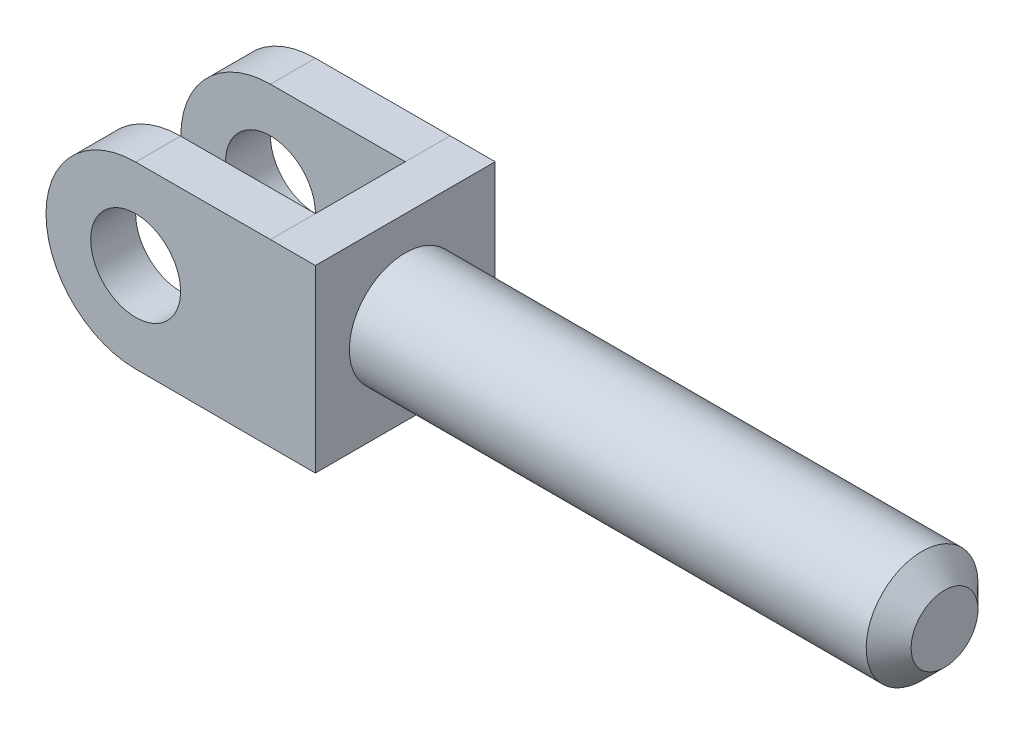
ISO-10303-21;
HEADER;
FILE_DESCRIPTION(('STEP AP214'),'2;1');
FILE_NAME('part.step','',(''),(''),'','','');
FILE_SCHEMA(('AUTOMOTIVE_DESIGN { 1 0 10303 214 1 1 1 1 }'));
ENDSEC;
DATA;
#1=APPLICATION_CONTEXT('core data for automotive mechanical design processes');
#2=APPLICATION_PROTOCOL_DEFINITION('international standard','automotive_design',2000,#1);
#3=PRODUCT_CONTEXT('',#1,'mechanical');
#4=PRODUCT('Part','Part','',(#3));
#5=PRODUCT_RELATED_PRODUCT_CATEGORY('part','',(#4));
#6=PRODUCT_DEFINITION_FORMATION('','',#4);
#7=PRODUCT_DEFINITION_CONTEXT('part definition',#1,'design');
#8=PRODUCT_DEFINITION('design','',#6,#7);
#9=PRODUCT_DEFINITION_SHAPE('','',#8);
#10=(LENGTH_UNIT() NAMED_UNIT(*) SI_UNIT(.MILLI.,.METRE.));
#11=(NAMED_UNIT(*) PLANE_ANGLE_UNIT() SI_UNIT($,.RADIAN.));
#12=(NAMED_UNIT(*) SI_UNIT($,.STERADIAN.) SOLID_ANGLE_UNIT());
#13=UNCERTAINTY_MEASURE_WITH_UNIT(LENGTH_MEASURE(1.E-05),#10,'distance_accuracy_value','');
#14=(GEOMETRIC_REPRESENTATION_CONTEXT(3) GLOBAL_UNCERTAINTY_ASSIGNED_CONTEXT((#13)) GLOBAL_UNIT_ASSIGNED_CONTEXT((#10,
#11,#12)) REPRESENTATION_CONTEXT('',''));
#15=CARTESIAN_POINT('',(0.,0.,0.));
#16=DIRECTION('',(0.,0.,1.));
#17=DIRECTION('',(1.,0.,0.));
#18=AXIS2_PLACEMENT_3D('',#15,#16,#17);
#19=CARTESIAN_POINT('',(0.,6.35,6.35));
#20=DIRECTION('',(1.,0.,0.));
#21=DIRECTION('',(0.,1.,0.));
#22=AXIS2_PLACEMENT_3D('',#19,#20,#21);
#23=PLANE('',#22);
#24=DIRECTION('',(0.,-1.,0.));
#25=VECTOR('',#24,1.);
#26=CARTESIAN_POINT('',(0.,6.35,3.175));
#27=LINE('',#26,#25);
#28=CARTESIAN_POINT('',(0.,6.35,3.175));
#29=VERTEX_POINT('',#28);
#30=CARTESIAN_POINT('',(0.,-6.35,3.175));
#31=VERTEX_POINT('',#30);
#32=EDGE_CURVE('E136',#29,#31,#27,.T.);
#33=ORIENTED_EDGE('',*,*,#32,.F.);
#34=DIRECTION('',(0.,0.,-1.));
#35=VECTOR('',#34,1.);
#36=CARTESIAN_POINT('',(0.,6.35,6.35));
#37=LINE('',#36,#35);
#38=CARTESIAN_POINT('',(0.,6.35,-3.175));
#39=VERTEX_POINT('',#38);
#40=EDGE_CURVE('E211',#29,#39,#37,.T.);
#41=ORIENTED_EDGE('',*,*,#40,.T.);
#42=DIRECTION('',(0.,-1.,0.));
#43=VECTOR('',#42,1.);
#44=CARTESIAN_POINT('',(0.,6.35,-3.175));
#45=LINE('',#44,#43);
#46=CARTESIAN_POINT('',(0.,-6.35,-3.175));
#47=VERTEX_POINT('',#46);
#48=EDGE_CURVE('E179',#39,#47,#45,.T.);
#49=ORIENTED_EDGE('',*,*,#48,.T.);
#50=DIRECTION('',(0.,0.,-1.));
#51=VECTOR('',#50,1.);
#52=CARTESIAN_POINT('',(0.,-6.35,6.35));
#53=LINE('',#52,#51);
#54=EDGE_CURVE('E60',#31,#47,#53,.T.);
#55=ORIENTED_EDGE('',*,*,#54,.F.);
#56=EDGE_LOOP('',(#33,#41,#49,#55));
#57=FACE_BOUND('',#56,.T.);
#58=ADVANCED_FACE('F41',(#57),#23,.F.);
#59=CARTESIAN_POINT('',(0.,-6.35,6.35));
#60=DIRECTION('',(0.,1.,0.));
#61=DIRECTION('',(0.,0.,1.));
#62=AXIS2_PLACEMENT_3D('',#59,#60,#61);
#63=PLANE('',#62);
#64=DIRECTION('',(1.,0.,0.));
#65=VECTOR('',#64,1.);
#66=CARTESIAN_POINT('',(0.,-6.35,-6.35));
#67=LINE('',#66,#65);
#68=CARTESIAN_POINT('',(0.,-6.35,-6.35));
#69=VERTEX_POINT('',#68);
#70=CARTESIAN_POINT('',(3.175,-6.35,-6.35));
#71=VERTEX_POINT('',#70);
#72=EDGE_CURVE('E192',#69,#71,#67,.T.);
#73=ORIENTED_EDGE('',*,*,#72,.T.);
#74=DIRECTION('',(0.,0.,-1.));
#75=VECTOR('',#74,1.);
#76=CARTESIAN_POINT('',(3.175,-6.35,6.35));
#77=LINE('',#76,#75);
#78=CARTESIAN_POINT('',(3.175,-6.35,6.35));
#79=VERTEX_POINT('',#78);
#80=EDGE_CURVE('E222',#79,#71,#77,.T.);
#81=ORIENTED_EDGE('',*,*,#80,.F.);
#82=DIRECTION('',(1.,0.,0.));
#83=VECTOR('',#82,1.);
#84=CARTESIAN_POINT('',(0.,-6.35,6.35));
#85=LINE('',#84,#83);
#86=CARTESIAN_POINT('',(0.,-6.35,6.35));
#87=VERTEX_POINT('',#86);
#88=EDGE_CURVE('E202',#87,#79,#85,.T.);
#89=ORIENTED_EDGE('',*,*,#88,.F.);
#90=EDGE_CURVE('E204',#87,#31,#53,.T.);
#91=ORIENTED_EDGE('',*,*,#90,.T.);
#92=ORIENTED_EDGE('',*,*,#54,.T.);
#93=DIRECTION('',(0.,0.,-1.));
#94=VECTOR('',#93,1.);
#95=CARTESIAN_POINT('',(0.,-6.35,-3.175));
#96=LINE('',#95,#94);
#97=EDGE_CURVE('E198',#47,#69,#96,.T.);
#98=ORIENTED_EDGE('',*,*,#97,.T.);
#99=EDGE_LOOP('',(#73,#81,#89,#91,#92,#98));
#100=FACE_BOUND('',#99,.T.);
#101=ADVANCED_FACE('F245',(#100),#63,.F.);
#102=CARTESIAN_POINT('',(3.175,6.35,6.35));
#103=DIRECTION('',(-1.,0.,0.));
#104=DIRECTION('',(0.,-1.,0.));
#105=AXIS2_PLACEMENT_3D('',#102,#103,#104);
#106=PLANE('',#105);
#107=CARTESIAN_POINT('',(3.175,0.,0.));
#108=DIRECTION('',(1.,0.,0.));
#109=DIRECTION('',(0.,1.,0.));
#110=AXIS2_PLACEMENT_3D('',#107,#108,#109);
#111=CIRCLE('',#110,3.95);
#112=CARTESIAN_POINT('',(3.175,-3.95,0.));
#113=VERTEX_POINT('',#112);
#114=EDGE_CURVE('E203',#113,#113,#111,.T.);
#115=ORIENTED_EDGE('',*,*,#114,.F.);
#116=EDGE_LOOP('',(#115));
#117=FACE_BOUND('',#116,.T.);
#118=DIRECTION('',(0.,1.,0.));
#119=VECTOR('',#118,1.);
#120=CARTESIAN_POINT('',(3.175,6.35,-6.35));
#121=LINE('',#120,#119);
#122=CARTESIAN_POINT('',(3.175,6.35,-6.35));
#123=VERTEX_POINT('',#122);
#124=EDGE_CURVE('E78',#71,#123,#121,.T.);
#125=ORIENTED_EDGE('',*,*,#124,.T.);
#126=DIRECTION('',(0.,0.,-1.));
#127=VECTOR('',#126,1.);
#128=CARTESIAN_POINT('',(3.175,6.35,6.35));
#129=LINE('',#128,#127);
#130=CARTESIAN_POINT('',(3.175,6.35,6.35));
#131=VERTEX_POINT('',#130);
#132=EDGE_CURVE('E218',#131,#123,#129,.T.);
#133=ORIENTED_EDGE('',*,*,#132,.F.);
#134=DIRECTION('',(0.,1.,0.));
#135=VECTOR('',#134,1.);
#136=CARTESIAN_POINT('',(3.175,6.35,6.35));
#137=LINE('',#136,#135);
#138=EDGE_CURVE('E68',#79,#131,#137,.T.);
#139=ORIENTED_EDGE('',*,*,#138,.F.);
#140=ORIENTED_EDGE('',*,*,#80,.T.);
#141=EDGE_LOOP('',(#125,#133,#139,#140));
#142=FACE_BOUND('',#141,.T.);
#143=ADVANCED_FACE('F249',(#117,#142),#106,.F.);
#144=CARTESIAN_POINT('',(0.,6.35,6.35));
#145=DIRECTION('',(0.,-1.,0.));
#146=DIRECTION('',(0.,0.,-1.));
#147=AXIS2_PLACEMENT_3D('',#144,#145,#146);
#148=PLANE('',#147);
#149=DIRECTION('',(-1.,0.,0.));
#150=VECTOR('',#149,1.);
#151=CARTESIAN_POINT('',(0.,6.35,-6.35));
#152=LINE('',#151,#150);
#153=CARTESIAN_POINT('',(0.,6.35,-6.35));
#154=VERTEX_POINT('',#153);
#155=EDGE_CURVE('E210',#123,#154,#152,.T.);
#156=ORIENTED_EDGE('',*,*,#155,.T.);
#157=DIRECTION('',(0.,0.,-1.));
#158=VECTOR('',#157,1.);
#159=CARTESIAN_POINT('',(0.,6.35,-3.175));
#160=LINE('',#159,#158);
#161=EDGE_CURVE('E196',#39,#154,#160,.T.);
#162=ORIENTED_EDGE('',*,*,#161,.F.);
#163=ORIENTED_EDGE('',*,*,#40,.F.);
#164=CARTESIAN_POINT('',(0.,6.35,6.35));
#165=VERTEX_POINT('',#164);
#166=EDGE_CURVE('E216',#165,#29,#37,.T.);
#167=ORIENTED_EDGE('',*,*,#166,.F.);
#168=DIRECTION('',(-1.,0.,0.));
#169=VECTOR('',#168,1.);
#170=CARTESIAN_POINT('',(0.,6.35,6.35));
#171=LINE('',#170,#169);
#172=EDGE_CURVE('E207',#131,#165,#171,.T.);
#173=ORIENTED_EDGE('',*,*,#172,.F.);
#174=ORIENTED_EDGE('',*,*,#132,.T.);
#175=EDGE_LOOP('',(#156,#162,#163,#167,#173,#174));
#176=FACE_BOUND('',#175,.T.);
#177=ADVANCED_FACE('F255',(#176),#148,.F.);
#178=CARTESIAN_POINT('',(0.,0.,6.35));
#179=DIRECTION('',(0.,0.,1.));
#180=DIRECTION('',(1.,0.,0.));
#181=AXIS2_PLACEMENT_3D('',#178,#179,#180);
#182=PLANE('',#181);
#183=ORIENTED_EDGE('',*,*,#172,.T.);
#184=DIRECTION('',(0.999998280209825,0.0018546097683996,0.));
#185=VECTOR('',#184,1.);
#186=CARTESIAN_POINT('',(-9.525,6.33233481157558,6.35));
#187=LINE('',#186,#185);
#188=CARTESIAN_POINT('',(-9.525,6.33233481157558,6.35));
#189=VERTEX_POINT('',#188);
#190=EDGE_CURVE('E151',#189,#165,#187,.T.);
#191=ORIENTED_EDGE('',*,*,#190,.F.);
#192=CARTESIAN_POINT('',(-9.525,0.,6.35));
#193=DIRECTION('',(0.,0.,-1.));
#194=DIRECTION('',(-1.,0.,0.));
#195=AXIS2_PLACEMENT_3D('',#192,#193,#194);
#196=CIRCLE('',#195,6.33233481157558);
#197=CARTESIAN_POINT('',(-9.525,-6.33233481157558,6.35));
#198=VERTEX_POINT('',#197);
#199=EDGE_CURVE('E159',#198,#189,#196,.T.);
#200=ORIENTED_EDGE('',*,*,#199,.F.);
#201=DIRECTION('',(-0.999998280209825,0.0018546097683996,0.));
#202=VECTOR('',#201,1.);
#203=CARTESIAN_POINT('',(-9.525,-6.33233481157558,6.35));
#204=LINE('',#203,#202);
#205=EDGE_CURVE('E82',#87,#198,#204,.T.);
#206=ORIENTED_EDGE('',*,*,#205,.F.);
#207=ORIENTED_EDGE('',*,*,#88,.T.);
#208=ORIENTED_EDGE('',*,*,#138,.T.);
#209=EDGE_LOOP('',(#183,#191,#200,#206,#207,#208));
#210=FACE_BOUND('',#209,.T.);
#211=CARTESIAN_POINT('',(-9.525,0.,6.35));
#212=DIRECTION('',(0.,0.,-1.));
#213=DIRECTION('',(-1.,0.,0.));
#214=AXIS2_PLACEMENT_3D('',#211,#212,#213);
#215=CIRCLE('',#214,3.175);
#216=CARTESIAN_POINT('',(-12.7,0.,6.35));
#217=VERTEX_POINT('',#216);
#218=EDGE_CURVE('E154',#217,#217,#215,.T.);
#219=ORIENTED_EDGE('',*,*,#218,.T.);
#220=EDGE_LOOP('',(#219));
#221=FACE_BOUND('',#220,.T.);
#222=ADVANCED_FACE('F256',(#210,#221),#182,.T.);
#223=CARTESIAN_POINT('',(0.,0.,-6.35));
#224=DIRECTION('',(0.,0.,1.));
#225=DIRECTION('',(1.,0.,0.));
#226=AXIS2_PLACEMENT_3D('',#223,#224,#225);
#227=PLANE('',#226);
#228=ORIENTED_EDGE('',*,*,#72,.F.);
#229=DIRECTION('',(-0.999998280209825,0.0018546097683996,0.));
#230=VECTOR('',#229,1.);
#231=CARTESIAN_POINT('',(-9.525,-6.33233481157558,-6.35));
#232=LINE('',#231,#230);
#233=CARTESIAN_POINT('',(-9.525,-6.33233481157558,-6.35));
#234=VERTEX_POINT('',#233);
#235=EDGE_CURVE('E178',#69,#234,#232,.T.);
#236=ORIENTED_EDGE('',*,*,#235,.T.);
#237=CARTESIAN_POINT('',(-9.525,0.,-6.35));
#238=DIRECTION('',(0.,0.,-1.));
#239=DIRECTION('',(-1.,0.,0.));
#240=AXIS2_PLACEMENT_3D('',#237,#238,#239);
#241=CIRCLE('',#240,6.33233481157558);
#242=CARTESIAN_POINT('',(-9.525,6.33233481157558,-6.35));
#243=VERTEX_POINT('',#242);
#244=EDGE_CURVE('E166',#234,#243,#241,.T.);
#245=ORIENTED_EDGE('',*,*,#244,.T.);
#246=DIRECTION('',(0.999998280209825,0.0018546097683996,0.));
#247=VECTOR('',#246,1.);
#248=CARTESIAN_POINT('',(-9.525,6.33233481157558,-6.35));
#249=LINE('',#248,#247);
#250=EDGE_CURVE('E190',#243,#154,#249,.T.);
#251=ORIENTED_EDGE('',*,*,#250,.T.);
#252=ORIENTED_EDGE('',*,*,#155,.F.);
#253=ORIENTED_EDGE('',*,*,#124,.F.);
#254=EDGE_LOOP('',(#228,#236,#245,#251,#252,#253));
#255=FACE_BOUND('',#254,.T.);
#256=CARTESIAN_POINT('',(-9.525,0.,-6.35));
#257=DIRECTION('',(0.,0.,-1.));
#258=DIRECTION('',(-1.,0.,0.));
#259=AXIS2_PLACEMENT_3D('',#256,#257,#258);
#260=CIRCLE('',#259,3.175);
#261=CARTESIAN_POINT('',(-12.7,0.,-6.35));
#262=VERTEX_POINT('',#261);
#263=EDGE_CURVE('E163',#262,#262,#260,.T.);
#264=ORIENTED_EDGE('',*,*,#263,.F.);
#265=EDGE_LOOP('',(#264));
#266=FACE_BOUND('',#265,.T.);
#267=ADVANCED_FACE('F257',(#255,#266),#227,.F.);
#268=CARTESIAN_POINT('',(41.275,0.,0.));
#269=DIRECTION('',(-1.,0.,0.));
#270=DIRECTION('',(0.,-1.,0.));
#271=AXIS2_PLACEMENT_3D('',#268,#269,#270);
#272=CYLINDRICAL_SURFACE('',#271,3.95);
#273=CARTESIAN_POINT('',(39.6875,0.,0.));
#274=DIRECTION('',(1.,0.,0.));
#275=DIRECTION('',(0.,1.,0.));
#276=AXIS2_PLACEMENT_3D('',#273,#274,#275);
#277=CIRCLE('',#276,3.95);
#278=CARTESIAN_POINT('',(39.6875,-3.95,0.));
#279=VERTEX_POINT('',#278);
#280=EDGE_CURVE('E11',#279,#279,#277,.F.);
#281=CARTESIAN_POINT('',(39.6875,-3.95,0.));
#282=CARTESIAN_POINT('',(39.3071614583334,-3.95,0.));
#283=CARTESIAN_POINT('',(38.9268229166667,-3.95,0.));
#284=CARTESIAN_POINT('',(38.1661458333334,-3.95,0.));
#285=CARTESIAN_POINT('',(37.7858072916667,-3.95,0.));
#286=CARTESIAN_POINT('',(37.0251302083334,-3.95,0.));
#287=CARTESIAN_POINT('',(36.6447916666667,-3.95,0.));
#288=CARTESIAN_POINT('',(35.8841145833334,-3.95,0.));
#289=CARTESIAN_POINT('',(35.5037760416667,-3.95,0.));
#290=CARTESIAN_POINT('',(34.7430989583334,-3.95,0.));
#291=CARTESIAN_POINT('',(34.3627604166667,-3.95,0.));
#292=CARTESIAN_POINT('',(33.6020833333334,-3.95,0.));
#293=CARTESIAN_POINT('',(33.2217447916667,-3.95,0.));
#294=CARTESIAN_POINT('',(32.4610677083334,-3.95,0.));
#295=CARTESIAN_POINT('',(32.0807291666667,-3.95,0.));
#296=CARTESIAN_POINT('',(31.3200520833334,-3.95,0.));
#297=CARTESIAN_POINT('',(30.9397135416667,-3.95,0.));
#298=CARTESIAN_POINT('',(30.1790364583334,-3.95,0.));
#299=CARTESIAN_POINT('',(29.7986979166667,-3.95,0.));
#300=CARTESIAN_POINT('',(29.0380208333334,-3.95,0.));
#301=CARTESIAN_POINT('',(28.6576822916667,-3.95,0.));
#302=CARTESIAN_POINT('',(27.8970052083334,-3.95,0.));
#303=CARTESIAN_POINT('',(27.5166666666667,-3.95,0.));
#304=CARTESIAN_POINT('',(26.7559895833334,-3.95,0.));
#305=CARTESIAN_POINT('',(26.3756510416667,-3.95,0.));
#306=CARTESIAN_POINT('',(25.6149739583334,-3.95,0.));
#307=CARTESIAN_POINT('',(25.2346354166667,-3.95,0.));
#308=CARTESIAN_POINT('',(24.4739583333334,-3.95,0.));
#309=CARTESIAN_POINT('',(24.0936197916667,-3.95,0.));
#310=CARTESIAN_POINT('',(23.3329427083334,-3.95,0.));
#311=CARTESIAN_POINT('',(22.9526041666667,-3.95,0.));
#312=CARTESIAN_POINT('',(22.1919270833334,-3.95,0.));
#313=CARTESIAN_POINT('',(21.8115885416667,-3.95,0.));
#314=CARTESIAN_POINT('',(21.0509114583334,-3.95,0.));
#315=CARTESIAN_POINT('',(20.6705729166667,-3.95,0.));
#316=CARTESIAN_POINT('',(19.9098958333334,-3.95,0.));
#317=CARTESIAN_POINT('',(19.5295572916667,-3.95,0.));
#318=CARTESIAN_POINT('',(18.7688802083333,-3.95,0.));
#319=CARTESIAN_POINT('',(18.3885416666667,-3.95,0.));
#320=CARTESIAN_POINT('',(17.6278645833334,-3.95,0.));
#321=CARTESIAN_POINT('',(17.2475260416667,-3.95,0.));
#322=CARTESIAN_POINT('',(16.4868489583333,-3.95,0.));
#323=CARTESIAN_POINT('',(16.1065104166667,-3.95,0.));
#324=CARTESIAN_POINT('',(15.3458333333333,-3.95,0.));
#325=CARTESIAN_POINT('',(14.9654947916667,-3.95,0.));
#326=CARTESIAN_POINT('',(14.2048177083333,-3.95,0.));
#327=CARTESIAN_POINT('',(13.8244791666667,-3.95,0.));
#328=CARTESIAN_POINT('',(13.0638020833333,-3.95,0.));
#329=CARTESIAN_POINT('',(12.6834635416667,-3.95,0.));
#330=CARTESIAN_POINT('',(11.9227864583333,-3.95,0.));
#331=CARTESIAN_POINT('',(11.5424479166667,-3.95,0.));
#332=CARTESIAN_POINT('',(10.7817708333333,-3.95,0.));
#333=CARTESIAN_POINT('',(10.4014322916667,-3.95,0.));
#334=CARTESIAN_POINT('',(9.64075520833334,-3.95,0.));
#335=CARTESIAN_POINT('',(9.26041666666668,-3.95,0.));
#336=CARTESIAN_POINT('',(8.49973958333335,-3.95,0.));
#337=CARTESIAN_POINT('',(8.11940104166668,-3.95,0.));
#338=CARTESIAN_POINT('',(7.35872395833334,-3.95,0.));
#339=CARTESIAN_POINT('',(6.97838541666667,-3.95,0.));
#340=CARTESIAN_POINT('',(6.21770833333334,-3.95,0.));
#341=CARTESIAN_POINT('',(5.83736979166668,-3.95,0.));
#342=CARTESIAN_POINT('',(5.07669270833335,-3.95,0.));
#343=CARTESIAN_POINT('',(4.69635416666668,-3.95,0.));
#344=CARTESIAN_POINT('',(3.93567708333334,-3.95,0.));
#345=CARTESIAN_POINT('',(3.55533854166667,-3.95,0.));
#346=CARTESIAN_POINT('',(3.175,-3.95,0.));
#347=B_SPLINE_CURVE_WITH_KNOTS('',3,(#281,#282,#283,#284,#285,#286,#287,#288,#289,#290,#291,
#292,#293,#294,#295,#296,#297,#298,#299,#300,#301,#302,#303,#304,#305,#306,#307,#308,#309,#310,
#311,#312,#313,#314,#315,#316,#317,#318,#319,#320,#321,#322,#323,#324,#325,#326,#327,#328,#329,
#330,#331,#332,#333,#334,#335,#336,#337,#338,#339,#340,#341,#342,#343,#344,#345,#346),
.UNSPECIFIED.,.F.,.F.,(4,2,2,2,2,2,2,2,2,2,2,2,2,2,2,2,2,2,2,2,2,2,2,2,2,2,2,2,2,2,2,2,4),(0.,
1.14101562500001,2.28203125,3.42304687500001,4.56406250000001,5.70507812500001,6.84609375000001,
7.98710937500001,9.12812500000001,10.269140625,11.41015625,12.551171875,13.6921875,14.833203125,
15.97421875,17.115234375,18.25625,19.397265625,20.53828125,21.679296875,22.8203125,23.961328125,
25.10234375,26.243359375,27.384375,28.525390625,29.66640625,30.807421875,31.9484375,
33.089453125,34.23046875,35.371484375,36.5125),.UNSPECIFIED.);
#348=EDGE_CURVE('BSEAM239',#279,#113,#347,.T.);
#349=ORIENTED_EDGE('',*,*,#280,.T.);
#350=ORIENTED_EDGE('',*,*,#114,.T.);
#351=ORIENTED_EDGE('',*,*,#348,.T.);
#352=ORIENTED_EDGE('',*,*,#348,.F.);
#353=EDGE_LOOP('',(#349,#351,#350,#352));
#354=FACE_BOUND('',#353,.T.);
#355=ADVANCED_FACE('F239',(#354),#272,.T.);
#356=CARTESIAN_POINT('',(41.275,0.,0.));
#357=DIRECTION('',(1.,0.,0.));
#358=DIRECTION('',(0.,1.,0.));
#359=AXIS2_PLACEMENT_3D('',#356,#357,#358);
#360=PLANE('',#359);
#361=CARTESIAN_POINT('',(41.275,0.,0.));
#362=DIRECTION('',(1.,0.,0.));
#363=DIRECTION('',(0.,1.,0.));
#364=AXIS2_PLACEMENT_3D('',#361,#362,#363);
#365=CIRCLE('',#364,2.36250000000003);
#366=CARTESIAN_POINT('',(41.275,2.36250000000003,0.));
#367=VERTEX_POINT('',#366);
#368=EDGE_CURVE('E49',#367,#367,#365,.T.);
#369=ORIENTED_EDGE('',*,*,#368,.T.);
#370=EDGE_LOOP('',(#369));
#371=FACE_BOUND('',#370,.T.);
#372=ADVANCED_FACE('F227',(#371),#360,.T.);
#373=CARTESIAN_POINT('',(41.275,0.,0.));
#374=DIRECTION('',(-1.,0.,0.));
#375=DIRECTION('',(0.,-1.,0.));
#376=AXIS2_PLACEMENT_3D('',#373,#374,#375);
#377=CONICAL_SURFACE('',#376,2.36250000000003,0.785398163397446);
#378=ORIENTED_EDGE('',*,*,#280,.F.);
#379=EDGE_LOOP('',(#378));
#380=FACE_BOUND('',#379,.T.);
#381=ORIENTED_EDGE('',*,*,#368,.F.);
#382=EDGE_LOOP('',(#381));
#383=FACE_BOUND('',#382,.T.);
#384=ADVANCED_FACE('F42',(#380,#383),#377,.T.);
#385=CARTESIAN_POINT('',(-9.525,0.,-3.175));
#386=DIRECTION('',(0.,0.,-1.));
#387=DIRECTION('',(-1.,0.,0.));
#388=AXIS2_PLACEMENT_3D('',#385,#386,#387);
#389=CYLINDRICAL_SURFACE('',#388,6.33233481157558);
#390=ORIENTED_EDGE('',*,*,#244,.F.);
#391=DIRECTION('',(0.,0.,-1.));
#392=VECTOR('',#391,1.);
#393=CARTESIAN_POINT('',(-9.525,-6.33233481157558,-3.175));
#394=LINE('',#393,#392);
#395=CARTESIAN_POINT('',(-9.525,-6.33233481157558,-3.175));
#396=VERTEX_POINT('',#395);
#397=EDGE_CURVE('E191',#396,#234,#394,.T.);
#398=ORIENTED_EDGE('',*,*,#397,.F.);
#399=CARTESIAN_POINT('',(-9.525,0.,-3.175));
#400=DIRECTION('',(0.,0.,-1.));
#401=DIRECTION('',(-1.,0.,0.));
#402=AXIS2_PLACEMENT_3D('',#399,#400,#401);
#403=CIRCLE('',#402,6.33233481157558);
#404=CARTESIAN_POINT('',(-9.525,6.33233481157558,-3.175));
#405=VERTEX_POINT('',#404);
#406=EDGE_CURVE('E174',#396,#405,#403,.T.);
#407=ORIENTED_EDGE('',*,*,#406,.T.);
#408=DIRECTION('',(0.,0.,-1.));
#409=VECTOR('',#408,1.);
#410=CARTESIAN_POINT('',(-9.525,6.33233481157558,-3.175));
#411=LINE('',#410,#409);
#412=EDGE_CURVE('E183',#405,#243,#411,.T.);
#413=ORIENTED_EDGE('',*,*,#412,.T.);
#414=EDGE_LOOP('',(#390,#398,#407,#413));
#415=FACE_BOUND('',#414,.T.);
#416=ADVANCED_FACE('F226',(#415),#389,.T.);
#417=CARTESIAN_POINT('',(-9.525,-6.33233481157558,-3.175));
#418=DIRECTION('',(-0.0018546097683996,-0.999998280209825,0.));
#419=DIRECTION('',(0.999998280209825,-0.0018546097683996,0.));
#420=AXIS2_PLACEMENT_3D('',#417,#418,#419);
#421=PLANE('',#420);
#422=ORIENTED_EDGE('',*,*,#235,.F.);
#423=ORIENTED_EDGE('',*,*,#97,.F.);
#424=DIRECTION('',(-0.999998280209825,0.0018546097683996,0.));
#425=VECTOR('',#424,1.);
#426=CARTESIAN_POINT('',(-9.525,-6.33233481157558,-3.175));
#427=LINE('',#426,#425);
#428=EDGE_CURVE('E185',#47,#396,#427,.T.);
#429=ORIENTED_EDGE('',*,*,#428,.T.);
#430=ORIENTED_EDGE('',*,*,#397,.T.);
#431=EDGE_LOOP('',(#422,#423,#429,#430));
#432=FACE_BOUND('',#431,.T.);
#433=ADVANCED_FACE('F237',(#432),#421,.T.);
#434=CARTESIAN_POINT('',(-9.525,6.33233481157558,-3.175));
#435=DIRECTION('',(-0.0018546097683996,0.999998280209825,0.));
#436=DIRECTION('',(-0.999998280209825,-0.0018546097683996,0.));
#437=AXIS2_PLACEMENT_3D('',#434,#435,#436);
#438=PLANE('',#437);
#439=ORIENTED_EDGE('',*,*,#250,.F.);
#440=ORIENTED_EDGE('',*,*,#412,.F.);
#441=DIRECTION('',(0.999998280209825,0.0018546097683996,0.));
#442=VECTOR('',#441,1.);
#443=CARTESIAN_POINT('',(-9.525,6.33233481157558,-3.175));
#444=LINE('',#443,#442);
#445=EDGE_CURVE('E173',#405,#39,#444,.T.);
#446=ORIENTED_EDGE('',*,*,#445,.T.);
#447=ORIENTED_EDGE('',*,*,#161,.T.);
#448=EDGE_LOOP('',(#439,#440,#446,#447));
#449=FACE_BOUND('',#448,.T.);
#450=ADVANCED_FACE('F268',(#449),#438,.T.);
#451=CARTESIAN_POINT('',(-9.525,0.,-3.175));
#452=DIRECTION('',(0.,0.,-1.));
#453=DIRECTION('',(-1.,0.,0.));
#454=AXIS2_PLACEMENT_3D('',#451,#452,#453);
#455=PLANE('',#454);
#456=CARTESIAN_POINT('',(-9.525,0.,-3.175));
#457=DIRECTION('',(0.,0.,-1.));
#458=DIRECTION('',(-1.,0.,0.));
#459=AXIS2_PLACEMENT_3D('',#456,#457,#458);
#460=CIRCLE('',#459,3.175);
#461=CARTESIAN_POINT('',(-12.7,0.,-3.175));
#462=VERTEX_POINT('',#461);
#463=EDGE_CURVE('E167',#462,#462,#460,.T.);
#464=ORIENTED_EDGE('',*,*,#463,.T.);
#465=EDGE_LOOP('',(#464));
#466=FACE_BOUND('',#465,.T.);
#467=ORIENTED_EDGE('',*,*,#406,.F.);
#468=ORIENTED_EDGE('',*,*,#428,.F.);
#469=ORIENTED_EDGE('',*,*,#48,.F.);
#470=ORIENTED_EDGE('',*,*,#445,.F.);
#471=EDGE_LOOP('',(#467,#468,#469,#470));
#472=FACE_BOUND('',#471,.T.);
#473=ADVANCED_FACE('F271',(#466,#472),#455,.F.);
#474=CARTESIAN_POINT('',(-9.525,0.,-3.175));
#475=DIRECTION('',(0.,0.,-1.));
#476=DIRECTION('',(-1.,0.,0.));
#477=AXIS2_PLACEMENT_3D('',#474,#475,#476);
#478=CYLINDRICAL_SURFACE('',#477,3.175);
#479=ORIENTED_EDGE('',*,*,#463,.F.);
#480=EDGE_LOOP('',(#479));
#481=FACE_BOUND('',#480,.T.);
#482=ORIENTED_EDGE('',*,*,#263,.T.);
#483=EDGE_LOOP('',(#482));
#484=FACE_BOUND('',#483,.T.);
#485=ADVANCED_FACE('F279',(#481,#484),#478,.F.);
#486=CARTESIAN_POINT('',(-9.525,0.,3.175));
#487=DIRECTION('',(0.,0.,1.));
#488=DIRECTION('',(-1.,0.,0.));
#489=AXIS2_PLACEMENT_3D('',#486,#487,#488);
#490=PLANE('',#489);
#491=CARTESIAN_POINT('',(-9.525,0.,3.175));
#492=DIRECTION('',(0.,0.,-1.));
#493=DIRECTION('',(-1.,0.,0.));
#494=AXIS2_PLACEMENT_3D('',#491,#492,#493);
#495=CIRCLE('',#494,6.33233481157558);
#496=CARTESIAN_POINT('',(-9.525,-6.33233481157558,3.175));
#497=VERTEX_POINT('',#496);
#498=CARTESIAN_POINT('',(-9.525,6.33233481157558,3.175));
#499=VERTEX_POINT('',#498);
#500=EDGE_CURVE('E133',#497,#499,#495,.T.);
#501=ORIENTED_EDGE('',*,*,#500,.T.);
#502=DIRECTION('',(0.999998280209825,0.0018546097683996,0.));
#503=VECTOR('',#502,1.);
#504=CARTESIAN_POINT('',(-9.525,6.33233481157558,3.175));
#505=LINE('',#504,#503);
#506=EDGE_CURVE('E150',#499,#29,#505,.T.);
#507=ORIENTED_EDGE('',*,*,#506,.T.);
#508=ORIENTED_EDGE('',*,*,#32,.T.);
#509=DIRECTION('',(-0.999998280209825,0.0018546097683996,0.));
#510=VECTOR('',#509,1.);
#511=CARTESIAN_POINT('',(-9.525,-6.33233481157558,3.175));
#512=LINE('',#511,#510);
#513=EDGE_CURVE('E128',#31,#497,#512,.T.);
#514=ORIENTED_EDGE('',*,*,#513,.T.);
#515=EDGE_LOOP('',(#501,#507,#508,#514));
#516=FACE_BOUND('',#515,.T.);
#517=CARTESIAN_POINT('',(-9.525,0.,3.175));
#518=DIRECTION('',(0.,0.,-1.));
#519=DIRECTION('',(-1.,0.,0.));
#520=AXIS2_PLACEMENT_3D('',#517,#518,#519);
#521=CIRCLE('',#520,3.175);
#522=CARTESIAN_POINT('',(-12.7,0.,3.175));
#523=VERTEX_POINT('',#522);
#524=EDGE_CURVE('E165',#523,#523,#521,.T.);
#525=ORIENTED_EDGE('',*,*,#524,.F.);
#526=EDGE_LOOP('',(#525));
#527=FACE_BOUND('',#526,.T.);
#528=ADVANCED_FACE('F134',(#516,#527),#490,.F.);
#529=CARTESIAN_POINT('',(-9.525,0.,3.175));
#530=DIRECTION('',(0.,0.,1.));
#531=DIRECTION('',(1.,0.,0.));
#532=AXIS2_PLACEMENT_3D('',#529,#530,#531);
#533=CYLINDRICAL_SURFACE('',#532,6.33233481157558);
#534=ORIENTED_EDGE('',*,*,#199,.T.);
#535=DIRECTION('',(0.,0.,1.));
#536=VECTOR('',#535,1.);
#537=CARTESIAN_POINT('',(-9.525,6.33233481157558,3.175));
#538=LINE('',#537,#536);
#539=EDGE_CURVE('E148',#499,#189,#538,.T.);
#540=ORIENTED_EDGE('',*,*,#539,.F.);
#541=ORIENTED_EDGE('',*,*,#500,.F.);
#542=DIRECTION('',(0.,0.,1.));
#543=VECTOR('',#542,1.);
#544=CARTESIAN_POINT('',(-9.525,-6.33233481157558,3.175));
#545=LINE('',#544,#543);
#546=EDGE_CURVE('E142',#497,#198,#545,.T.);
#547=ORIENTED_EDGE('',*,*,#546,.T.);
#548=EDGE_LOOP('',(#534,#540,#541,#547));
#549=FACE_BOUND('',#548,.T.);
#550=ADVANCED_FACE('F149',(#549),#533,.T.);
#551=CARTESIAN_POINT('',(-9.525,6.33233481157558,3.175));
#552=DIRECTION('',(0.0018546097683996,-0.999998280209825,0.));
#553=DIRECTION('',(0.999998280209825,0.0018546097683996,0.));
#554=AXIS2_PLACEMENT_3D('',#551,#552,#553);
#555=PLANE('',#554);
#556=ORIENTED_EDGE('',*,*,#190,.T.);
#557=ORIENTED_EDGE('',*,*,#166,.T.);
#558=ORIENTED_EDGE('',*,*,#506,.F.);
#559=ORIENTED_EDGE('',*,*,#539,.T.);
#560=EDGE_LOOP('',(#556,#557,#558,#559));
#561=FACE_BOUND('',#560,.T.);
#562=ADVANCED_FACE('F281',(#561),#555,.F.);
#563=CARTESIAN_POINT('',(-9.525,-6.33233481157558,3.175));
#564=DIRECTION('',(0.0018546097683996,0.999998280209825,0.));
#565=DIRECTION('',(-0.999998280209825,0.0018546097683996,0.));
#566=AXIS2_PLACEMENT_3D('',#563,#564,#565);
#567=PLANE('',#566);
#568=ORIENTED_EDGE('',*,*,#205,.T.);
#569=ORIENTED_EDGE('',*,*,#546,.F.);
#570=ORIENTED_EDGE('',*,*,#513,.F.);
#571=ORIENTED_EDGE('',*,*,#90,.F.);
#572=EDGE_LOOP('',(#568,#569,#570,#571));
#573=FACE_BOUND('',#572,.T.);
#574=ADVANCED_FACE('F141',(#573),#567,.F.);
#575=CARTESIAN_POINT('',(-9.525,0.,3.175));
#576=DIRECTION('',(0.,0.,1.));
#577=DIRECTION('',(1.,0.,0.));
#578=AXIS2_PLACEMENT_3D('',#575,#576,#577);
#579=CYLINDRICAL_SURFACE('',#578,3.175);
#580=ORIENTED_EDGE('',*,*,#524,.T.);
#581=EDGE_LOOP('',(#580));
#582=FACE_BOUND('',#581,.T.);
#583=ORIENTED_EDGE('',*,*,#218,.F.);
#584=EDGE_LOOP('',(#583));
#585=FACE_BOUND('',#584,.T.);
#586=ADVANCED_FACE('F290',(#582,#585),#579,.F.);
#587=CLOSED_SHELL('',(#58,#101,#143,#177,#222,#267,#355,#372,#384,#416,#433,#450,#473,#485,#528,
#550,#562,#574,#586));
#588=MANIFOLD_SOLID_BREP('B2',#587);
#589=ADVANCED_BREP_SHAPE_REPRESENTATION('',(#18,#588),#14);
#590=SHAPE_DEFINITION_REPRESENTATION(#9,#589);
ENDSEC;
END-ISO-10303-21;
